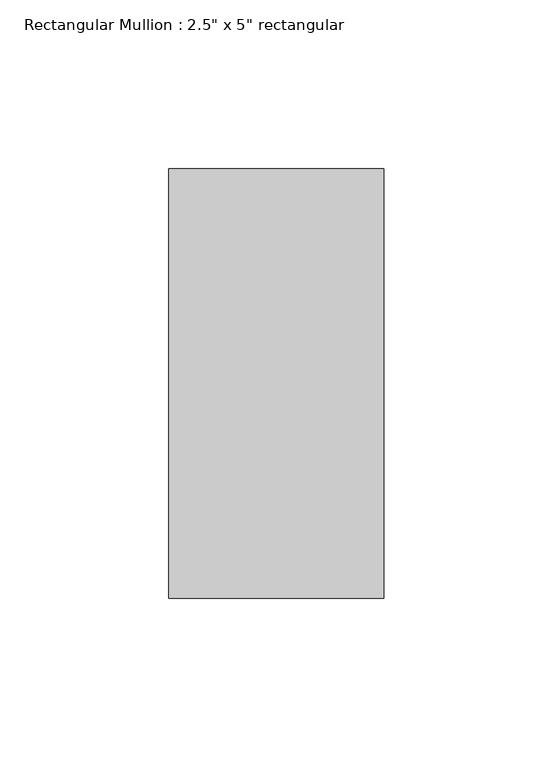
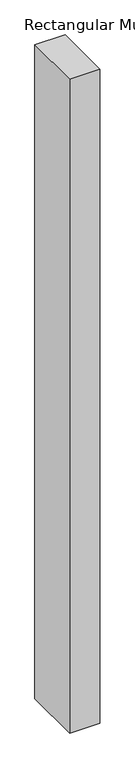
"""IFC4 building model written with IfcOpenShell, lengths in millimetres: member geometry."""

from ifc_helpers import new_model, si_unit, frame, origin, place, context, project, spatial, polyline, outline, extrude, source, transform, mapped, element, save


def member_d9285493(model_context):
    return source(origin(), model_context, "Body", "SweptSolid", [
        extrude(outline(polyline([(31.75, 63.5), (31.75, -63.5), (-31.75, -63.5), (-31.75, 63.5), (31.75, 63.5)])), frame((0.0, 0.0, -1457.6985165), z_axis=(0.0, 0.0, 1.0), x_axis=(1.0, 0.0, 0.0)), (0.0, 0.0, 1.0), 1457.6985165),
    ])


if __name__ == "__main__":
    model = new_model("IFC4")
    model_context = context("Model", 3, world=origin())
    ifc_project = project(units=[si_unit("LENGTHUNIT", "METRE", prefix="MILLI")], contexts=[model_context])
    site = spatial("IfcSite", under=ifc_project)
    building = spatial("IfcBuilding", under=site)
    placement = place(None, origin())
    member_shape = member_d9285493(model_context)
    element("IfcMember", 1, ObjectType="Rectangular Mullion : 2.5\" x 5\" rectangular", at=placement, inside=building, context=model_context, shape_type="MappedRepresentation", body=[
        mapped(member_shape, transform((0.0, 0.0, 0.0), x_axis=(1.0, 0.0, 0.0), y_axis=(0.0, 1.0, 0.0), z_axis=(0.0, 0.0, 1.0))),
    ])
    save(model, "model.ifc")

# Revit data of these elements
# Type "Rectangular Mullion : 2.5\" x 5\" rectangular"
#   built-in parameter 1007304 = 0.416667 (stored number, unit not read)
#   built-in parameter 1007301 = 0.104167 (stored number, unit not read)
#   built-in parameter 1007300 = 0.104167 (stored number, unit not read)
# Element 1 (IfcMember, "Rectangular Mullion : 2.5\" x 5\" rectangular")
#   Materials on its faces: "Aluminum"
# Materials
#   "Aluminum": class "Metal", colour RGB 247 247 247, transparency 0, Description = "Aluminum 6061", Cost = 0
